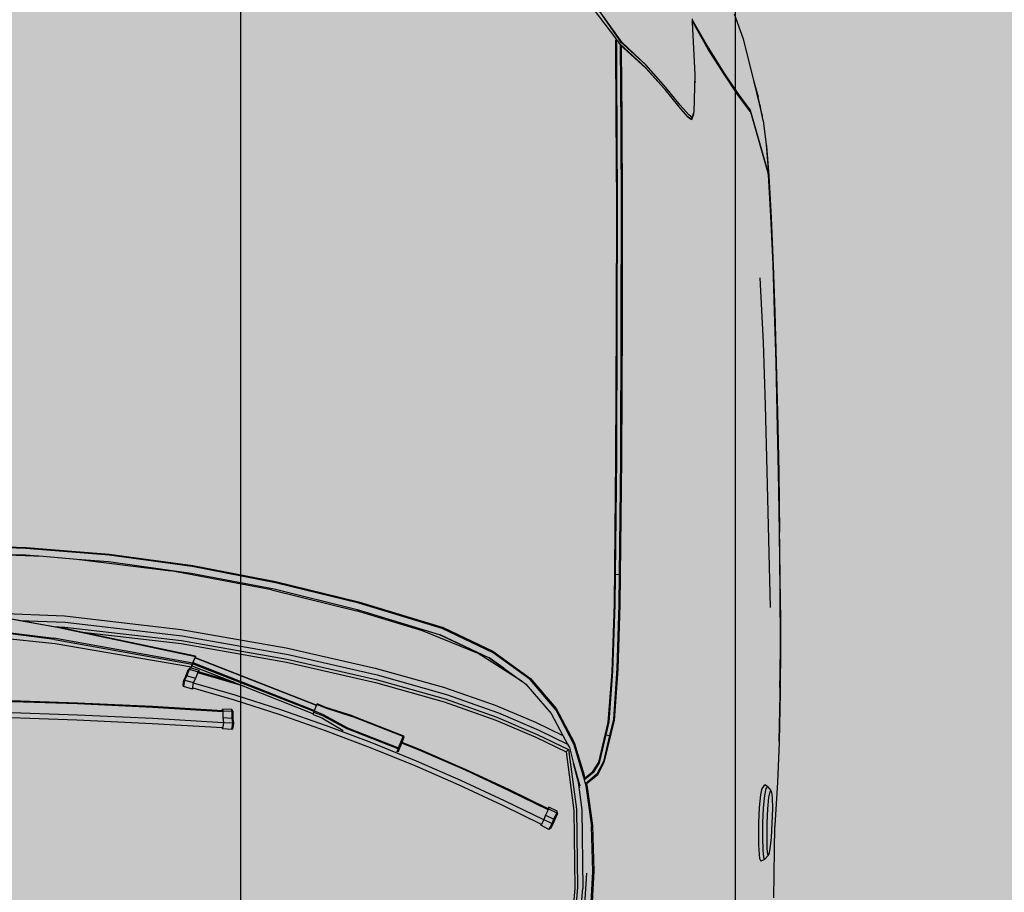
# Model space of a CAD drawing. Units: inches. Extents: x 1884 to 2398, y 474 to 1488.
# Tile 17 of 39: x 2233 to 2275, y 699 to 736. Entities that reach past the tile are written whole.
import ezdxf

# ---------------------------------------------------------------- set-up
doc = ezdxf.new("R2010")
doc.units = ezdxf.units.IN
doc.header["$MEASUREMENT"] = 0
doc.layers.get('0').update_dxf_attribs({"color": 250})
doc.layers.add('A-ANNO-DIMS', color=2, linetype='Continuous', lineweight=18)
doc.layers.add('C-VEHI', color=8, linetype='Continuous', lineweight=18)
doc.layers.add('Edges', color=250, linetype='Continuous')
doc.layers.add('L-PVMT-PATT', color=9, linetype='Continuous', lineweight=13, true_color=0xc7c8ca)
doc.styles.get("Standard").update_dxf_attribs({"font": 'arial.ttf'})
doc.dimstyles.get("Standard").update_dxf_attribs({"dimtxt": 7, "dimasz": 0.18, "dimexe": 0.18, "dimexo": 0.0625, "dimgap": 0.09, "dimtad": 0, "dimtih": 1, "dimtoh": 1, "dimzin": 0, "dimdsep": 46, "dimlunit": 3, "dimtxsty": 'Standard', "dimcen": 0.09, "dimadec": 0, "dimazin": 0, "dimtfac": 1, "dimtofl": 0, "dimtmove": 0, "dimatfit": 3, "dimfxl": 1, "dimtolj": 1, "dimtzin": 0, "dimarcsym": 0})

# ---------------------------------------------------------------- blocks, each defined once
blk = doc.blocks.new('Nissan Qashqai pl')
at = {"layer": 'Edges'}
for p, q in [((8.0713, 12.8205), (8.016, 12.8189)), ((8.0168, 12.8191), (8.0718, 12.8207)), ((8.1249, 12.8218), (8.0713, 12.8205)), ((8.0718, 12.8207), (8.1251, 12.822)), ((8.1901, 12.8232), (8.1249, 12.8218)), ((8.1251, 12.822), (8.1902, 12.8233)), ((8.2094, 12.8235), (8.1901, 12.8232)), ((8.1902, 12.8233), (8.2543, 12.8243)), ((8.2543, 12.8243), (8.2094, 12.8235)), ((8.2543, 12.8243), (8.2094, 12.8235)), ((8.2544, 12.8242), (8.2094, 12.8235)), ((8.2693, 12.8245), (8.2543, 12.8243)), ((8.3166, 12.8249), (8.2544, 12.8242)), ((8.3098, 12.825), (8.2693, 12.8245)), ((8.3159, 12.825), (8.2693, 12.8245)), ((8.3159, 12.825), (8.3098, 12.825)), ((8.3159, 12.825), (8.3163, 12.825)), ((8.3163, 12.825), (8.3657, 12.8252)), ((8.3163, 12.825), (8.3597, 12.8252)), ((8.3764, 12.8251), (8.3166, 12.8249)), ((8.3597, 12.8252), (8.3657, 12.8252)), ((8.3657, 12.8252), (8.3663, 12.8252)), ((8.3663, 12.8252), (8.3747, 12.8252)), ((8.3764, 12.8251), (8.3663, 12.8252)), ((8.3747, 12.8252), (8.3757, 12.8252)), ((8.3757, 12.8252), (8.4282, 12.8249)), ((8.4069, 12.8249), (8.3764, 12.8251)), ((8.4219, 12.8246), (8.4069, 12.8249)), ((8.4292, 12.8248), (8.4069, 12.8249)), ((8.4282, 12.8249), (8.4799, 12.8239)), ((8.4799, 12.8239), (8.4292, 12.8248)), ((8.4799, 12.8239), (8.4811, 12.8239)), ((8.4811, 12.8239), (8.5241, 12.8222)), ((8.5241, 12.8222), (8.5707, 12.8193)), ((7.8676, 12.8123), (7.7998, 12.7928)), ((7.8012, 12.7929), (7.8681, 12.8121)), ((7.8107, 12.8065), (7.8363, 12.8097)), ((7.8363, 12.8097), (7.8676, 12.8123)), ((7.8363, 12.8097), (7.8381, 12.81)), ((7.8381, 12.81), (7.87, 12.8126)), ((7.8676, 12.8123), (7.8681, 12.8121)), ((7.869, 12.8124), (7.8681, 12.8121)), ((7.9137, 12.815), (7.869, 12.8124)), ((7.87, 12.8126), (7.9151, 12.8152)), ((7.9658, 12.8172), (7.9137, 12.815)), ((7.9151, 12.8152), (7.9668, 12.8174)), ((8.016, 12.8189), (7.9658, 12.8172)), ((7.9668, 12.8174), (8.0168, 12.8191)), ((8.1176, 12.8087), (8.1888, 12.8107)), ((8.1888, 12.8107), (8.2622, 12.8125)), ((8.2622, 12.8125), (8.3356, 12.8141)), ((8.5287, 12.8112), (8.5269, 12.8082)), ((8.5287, 12.8112), (8.5331, 12.815)), ((8.5287, 12.8112), (8.531, 12.8095)), ((8.5347, 12.8159), (8.5331, 12.815)), ((8.5331, 12.815), (8.5346, 12.8138)), ((8.5346, 12.8138), (8.5406, 12.8125)), ((8.5407, 12.8167), (8.5347, 12.8159)), ((8.5406, 12.8125), (8.5526, 12.8114)), ((8.5527, 12.8169), (8.5407, 12.8167)), ((8.5526, 12.8114), (8.5681, 12.8107)), ((8.5682, 12.8164), (8.5527, 12.8169)), ((8.5681, 12.8107), (8.5836, 12.8104)), ((8.5837, 12.8154), (8.5682, 12.8164)), ((8.5707, 12.8193), (8.5719, 12.8193)), ((8.6489, 12.8179), (8.5719, 12.8193)), ((8.5836, 12.8104), (8.5957, 12.8107)), ((8.5958, 12.8141), (8.5837, 12.8154)), ((8.5957, 12.8107), (8.6017, 12.8114)), ((8.6018, 12.8129), (8.5958, 12.8141)), ((8.6017, 12.8114), (8.6032, 12.8121)), ((8.6032, 12.8121), (8.6018, 12.8129)), ((8.6073, 12.808), (8.6032, 12.8121)), ((7.7673, 12.7961), (7.8058, 12.8055)), ((7.7673, 12.7961), (7.7848, 12.8012)), ((7.7835, 12.8007), (7.7835, 12.8007)), ((7.8087, 12.8062), (7.7848, 12.8012)), ((7.7865, 12.8013), (7.7866, 12.8013)), ((7.7936, 12.8029), (7.7977, 12.8038)), ((7.8106, 12.8065), (7.8087, 12.8062)), ((7.8106, 12.8065), (7.8107, 12.8065)), ((7.9803, 12.803), (8.05, 12.8066)), ((8.05, 12.8066), (8.1176, 12.8087)), ((8.5322, 12.8047), (8.5269, 12.8082)), ((8.531, 12.8095), (8.5385, 12.8079)), ((8.5322, 12.8047), (8.5375, 12.8036)), ((8.5375, 12.8036), (8.5513, 12.8023)), ((8.5385, 12.8079), (8.5518, 12.8066)), ((8.5513, 12.8023), (8.5678, 12.8016)), ((8.5518, 12.8066), (8.568, 12.8059)), ((8.5678, 12.8016), (8.5844, 12.8014)), ((8.568, 12.8059), (8.5842, 12.8057)), ((8.5842, 12.8057), (8.5974, 12.8061)), ((8.5844, 12.8014), (8.5921, 12.8016)), ((8.5921, 12.8016), (8.6021, 12.8022)), ((8.5974, 12.8061), (8.6049, 12.8069)), ((8.6021, 12.8022), (8.6065, 12.8027)), ((8.6049, 12.8069), (8.6073, 12.808)), ((8.6065, 12.8027), (8.6093, 12.804)), ((8.6073, 12.808), (8.6093, 12.804)), ((7.7223, 12.7851), (7.7673, 12.7961)), ((7.7814, 12.7791), (7.7991, 12.7923)), ((7.7984, 12.7909), (7.7828, 12.7793)), ((7.7976, 12.792), (7.7991, 12.7923)), ((7.8007, 12.7926), (7.7984, 12.7909)), ((7.7991, 12.7923), (7.7998, 12.7928)), ((7.7995, 12.7924), (7.8007, 12.7926)), ((7.8012, 12.7929), (7.8007, 12.7926)), ((7.6953, 12.7753), (7.7223, 12.7851)), ((7.7591, 12.7641), (7.7814, 12.7791)), ((7.7828, 12.7793), (7.7606, 12.7644)), ((7.7325, 12.7476), (7.7591, 12.7641)), ((7.7606, 12.7644), (7.7341, 12.7478)), ((7.7038, 12.731), (7.7325, 12.7476)), ((7.7341, 12.7478), (7.7056, 12.7314)), ((7.701, 12.73), (7.7024, 12.7301)), ((7.7024, 12.7301), (7.7038, 12.731)), ((7.7024, 12.7301), (7.7034, 12.7301)), ((7.7056, 12.7314), (7.7034, 12.7301)), ((7.7034, 12.7301), (7.7048, 12.7302)), ((7.7048, 12.7302), (7.7608, 12.7329)), ((7.7058, 12.7308), (7.7048, 12.7302)), ((7.7608, 12.7329), (7.8014, 12.7318)), ((7.7688, 12.7328), (7.7688, 12.734)), ((7.8045, 12.7263), (7.7938, 12.7171)), ((7.8062, 12.725), (7.7959, 12.7161)), ((7.8014, 12.7318), (7.8022, 12.7316)), ((7.8022, 12.7316), (7.8037, 12.7315)), ((7.8022, 12.7316), (7.8072, 12.73)), ((7.8037, 12.7315), (7.8096, 12.7294)), ((7.8072, 12.73), (7.8045, 12.7263)), ((7.8062, 12.725), (7.8087, 12.7283)), ((7.8066, 12.7254), (7.8062, 12.725)), ((7.8096, 12.7294), (7.8066, 12.7254)), ((7.8072, 12.73), (7.8087, 12.7283)), ((7.7938, 12.7171), (7.7748, 12.7018)), ((7.7959, 12.7161), (7.7772, 12.7011)), ((7.7748, 12.7018), (7.7507, 12.6803)), ((7.753, 12.6794), (7.776, 12.6999)), ((7.776, 12.6999), (7.7539, 12.68)), ((7.7772, 12.7011), (7.776, 12.6999)), ((7.7261, 12.6543), (7.7507, 12.6803)), ((7.753, 12.6794), (7.7281, 12.6524)), ((7.7507, 12.6803), (7.7286, 12.6561)), ((7.7539, 12.68), (7.7324, 12.6565)), ((7.7261, 12.6543), (7.6762, 12.6186)), ((7.6762, 12.6186), (7.7233, 12.6514)), ((7.7281, 12.6524), (7.7232, 12.6486)), ((7.7267, 12.6539), (7.7233, 12.6514)), ((7.7286, 12.6561), (7.7267, 12.6539)), ((7.7299, 12.6537), (7.7281, 12.6524)), ((7.7281, 12.6524), (7.7349, 12.6524)), ((7.7324, 12.6565), (7.7299, 12.6537)), ((7.7299, 12.6537), (7.7334, 12.6537)), ((7.7334, 12.6537), (7.8083, 12.6544)), ((7.7349, 12.6524), (7.768, 12.6527)), ((7.768, 12.6527), (7.7692, 12.6527)), ((7.7692, 12.6527), (7.7844, 12.6528)), ((7.7844, 12.6528), (7.8078, 12.653)), ((7.8078, 12.653), (7.8233, 12.6531)), ((7.8083, 12.6544), (7.904, 12.6547)), ((7.8233, 12.6531), (7.9036, 12.6534)), ((7.9036, 12.6534), (8.0275, 12.6533)), ((7.904, 12.6547), (8.0276, 12.6545)), ((8.0275, 12.6533), (8.1755, 12.6527)), ((8.0276, 12.6545), (8.1753, 12.6539)), ((8.1753, 12.6539), (8.3324, 12.6521)), ((8.1755, 12.6527), (8.3005, 12.6514)), ((8.3005, 12.6514), (8.3002, 12.6474)), ((8.3005, 12.6514), (8.3324, 12.651)), ((8.3324, 12.6521), (8.4022, 12.6498)), ((8.3324, 12.651), (8.4014, 12.6488)), ((7.6771, 12.6135), (7.7215, 12.6473)), ((7.7215, 12.6473), (7.7221, 12.6478)), ((7.7232, 12.6486), (7.7221, 12.6478)), ((7.7245, 12.6486), (7.7232, 12.6486)), ((7.7261, 12.6476), (7.7238, 12.6476)), ((7.7294, 12.6487), (7.7245, 12.6486)), ((7.7279, 12.6477), (7.7261, 12.6476)), ((7.8048, 12.6483), (7.7279, 12.6477)), ((7.731, 12.6487), (7.7294, 12.6487)), ((7.764, 12.6489), (7.731, 12.6487)), ((7.7662, 12.6489), (7.764, 12.6489)), ((7.7811, 12.649), (7.7662, 12.6489)), ((7.7822, 12.649), (7.7811, 12.649)), ((7.8057, 12.6491), (7.7822, 12.649)), ((7.9014, 12.6487), (7.8048, 12.6483)), ((7.8233, 12.6492), (7.8057, 12.6491)), ((7.902, 12.6495), (7.8233, 12.6492)), ((8.0273, 12.6485), (7.9014, 12.6487)), ((8.0275, 12.6493), (7.902, 12.6495)), ((8.1753, 12.6479), (8.0273, 12.6485)), ((8.1754, 12.6487), (8.0275, 12.6493)), ((8.3318, 12.6462), (8.1753, 12.6479)), ((8.3002, 12.6474), (8.1754, 12.6487)), ((8.332, 12.6471), (8.3002, 12.6474)), ((8.4049, 12.6437), (8.3318, 12.6462)), ((8.4042, 12.6447), (8.332, 12.6471)), ((8.4014, 12.6488), (8.4559, 12.6451)), ((8.4022, 12.6498), (8.4571, 12.6459)), ((8.4588, 12.6405), (8.4042, 12.6447)), ((8.4595, 12.6395), (8.4049, 12.6437)), ((8.4559, 12.6451), (8.4736, 12.6409)), ((8.4571, 12.6459), (8.5029, 12.635)), ((8.4729, 12.6372), (8.4588, 12.6405)), ((8.4729, 12.6372), (8.4736, 12.6409)), ((8.4736, 12.6409), (8.5018, 12.6344)), ((8.5025, 12.6293), (8.4595, 12.6395)), ((8.5032, 12.6301), (8.4729, 12.6372)), ((8.5018, 12.6344), (8.5155, 12.6274)), ((8.5125, 12.6231), (8.5025, 12.6293)), ((8.5029, 12.635), (8.5163, 12.6279)), ((8.5132, 12.624), (8.5032, 12.6301)), ((8.5177, 12.617), (8.5125, 12.6231)), ((8.5132, 12.624), (8.5216, 12.6139)), ((8.5155, 12.6274), (8.5258, 12.6151)), ((8.5163, 12.6279), (8.5237, 12.6189)), ((8.5237, 12.6189), (8.5259, 12.6162)), ((8.5294, 12.6167), (8.5706, 12.6226)), ((8.5304, 12.6157), (8.5715, 12.6215)), ((8.5706, 12.6226), (8.6197, 12.6241)), ((8.6203, 12.6229), (8.5715, 12.6215)), ((8.6197, 12.6241), (8.6683, 12.6215)), ((8.6203, 12.6229), (8.6204, 12.6229)), ((8.6721, 12.6201), (8.6204, 12.6229)), ((8.4814, 12.6029), (8.5166, 12.6135)), ((8.5216, 12.6139), (8.4838, 12.6027)), ((8.5039, 12.6023), (8.528, 12.6088)), ((8.5166, 12.6135), (8.5197, 12.6145)), ((8.5197, 12.6145), (8.5177, 12.617)), ((8.5197, 12.6145), (8.5216, 12.6139)), ((8.5258, 12.6151), (8.5216, 12.6139)), ((8.5216, 12.6068), (8.5538, 12.6111)), ((8.5301, 12.609), (8.5216, 12.6068)), ((8.5259, 12.6162), (8.5258, 12.6151)), ((8.5258, 12.6151), (8.5304, 12.6157)), ((8.5259, 12.6162), (8.5294, 12.6167)), ((8.5304, 12.6157), (8.5304, 12.6157)), ((8.5538, 12.6111), (8.6387, 12.6123)), ((8.622, 12.6161), (8.6699, 12.6132)), ((8.6721, 12.6093), (8.6387, 12.6123)), ((8.4444, 12.5834), (8.4814, 12.6029)), ((8.4838, 12.6027), (8.4462, 12.5833)), ((8.4831, 12.5957), (8.4867, 12.5977)), ((8.4867, 12.5977), (8.5039, 12.6023)), ((8.4889, 12.5969), (8.5531, 12.6055)), ((8.4914, 12.5942), (8.5544, 12.6026)), ((8.5216, 12.6068), (8.5039, 12.6023)), ((8.5531, 12.6055), (8.6375, 12.6066)), ((8.5544, 12.6026), (8.6386, 12.6037)), ((8.6375, 12.6066), (8.7481, 12.5968)), ((8.6386, 12.6037), (8.7491, 12.594)), ((8.4499, 12.5782), (8.4737, 12.5908)), ((8.4594, 12.5611), (8.4737, 12.5908)), ((8.468, 12.5648), (8.4831, 12.5957)), ((8.4725, 12.563), (8.4889, 12.5969)), ((8.4737, 12.5908), (8.4831, 12.5957)), ((8.4756, 12.5615), (8.4914, 12.5942)), ((8.4914, 12.5942), (8.4889, 12.5969)), ((8.4122, 12.5558), (8.4444, 12.5834)), ((8.4462, 12.5833), (8.4134, 12.5554)), ((8.4183, 12.5508), (8.4499, 12.5782)), ((8.5554, 12.5847), (8.551, 12.5757)), ((8.5529, 12.5751), (8.5572, 12.5841)), ((8.5574, 12.5849), (8.5554, 12.5847)), ((8.5572, 12.5841), (8.5554, 12.5847)), ((8.5639, 12.581), (8.5572, 12.5841)), ((8.5574, 12.5849), (8.5584, 12.5846)), ((8.5582, 12.5845), (8.5574, 12.5849)), ((8.5584, 12.5846), (8.5649, 12.5816)), ((8.5595, 12.572), (8.5639, 12.581)), ((8.5687, 12.5791), (8.5639, 12.581)), ((8.5644, 12.5701), (8.5687, 12.5791)), ((8.5649, 12.5816), (8.5693, 12.5799)), ((8.5687, 12.5791), (8.5693, 12.5799)), ((8.5749, 12.5757), (8.5687, 12.5791)), ((8.5693, 12.5799), (8.5739, 12.5774)), ((8.5739, 12.5774), (8.5749, 12.5757)), ((8.5527, 12.5749), (8.5323, 12.5332)), ((8.5537, 12.5747), (8.5332, 12.5329)), ((8.5647, 12.57), (8.5441, 12.5279)), ((8.5487, 12.5256), (8.5692, 12.5674)), ((8.5527, 12.5749), (8.551, 12.5757)), ((8.551, 12.5757), (8.5528, 12.5751)), ((8.5528, 12.5751), (8.5527, 12.5749)), ((8.5528, 12.5751), (8.5529, 12.5751)), ((8.5529, 12.5751), (8.5537, 12.5747)), ((8.5537, 12.5747), (8.5595, 12.572)), ((8.5595, 12.572), (8.5644, 12.5701)), ((8.5644, 12.5701), (8.5647, 12.57)), ((8.5647, 12.57), (8.5692, 12.5675)), ((8.5692, 12.5674), (8.5692, 12.5675)), ((8.5692, 12.5675), (8.5705, 12.5668)), ((8.5705, 12.5668), (8.5692, 12.5674)), ((8.5749, 12.5757), (8.5705, 12.5668)), ((8.3826, 12.5151), (8.4122, 12.5558)), ((8.4134, 12.5554), (8.3844, 12.5157)), ((8.4411, 12.5178), (8.4594, 12.5611)), ((8.4493, 12.5212), (8.468, 12.5648)), ((8.454, 12.5196), (8.4725, 12.563)), ((8.4571, 12.5184), (8.4756, 12.5615)), ((8.4154, 12.5468), (8.3852, 12.4994)), ((8.3901, 12.5113), (8.4154, 12.5468)), ((8.4011, 12.5269), (8.4154, 12.5468)), ((8.4156, 12.547), (8.4154, 12.5468)), ((8.4156, 12.547), (8.4183, 12.5508)), ((8.4011, 12.5269), (8.3901, 12.5113)), ((8.3904, 12.512), (8.4011, 12.5269)), ((8.5323, 12.5332), (8.5103, 12.4859)), ((8.5332, 12.5329), (8.5112, 12.4856)), ((8.5441, 12.5279), (8.5222, 12.4807)), ((8.5269, 12.4785), (8.5487, 12.5256)), ((8.3573, 12.4618), (8.3826, 12.5151)), ((8.3844, 12.5157), (8.3582, 12.4606)), ((8.4217, 12.4622), (8.4411, 12.5178)), ((8.4296, 12.4651), (8.4493, 12.5212)), ((8.4343, 12.4637), (8.454, 12.5196)), ((8.4375, 12.4627), (8.4571, 12.5184)), ((8.3646, 12.4572), (8.39, 12.5111)), ((8.3648, 12.4579), (8.39, 12.5111)), ((8.39, 12.5111), (8.3852, 12.4994)), ((8.39, 12.5111), (8.3901, 12.5113)), ((8.3901, 12.5113), (8.3904, 12.512)), ((8.3852, 12.4994), (8.3608, 12.4393)), ((8.5103, 12.4859), (8.4895, 12.4381)), ((8.5112, 12.4856), (8.4904, 12.4377)), ((8.5222, 12.4807), (8.5014, 12.4329)), ((8.5062, 12.431), (8.5269, 12.4785)), ((8.3296, 12.3703), (8.3573, 12.4618)), ((8.3582, 12.4606), (8.3311, 12.3708)), ((8.4009, 12.3883), (8.4217, 12.4622)), ((8.4084, 12.3907), (8.4296, 12.4651)), ((8.4133, 12.3896), (8.4343, 12.4637)), ((8.4165, 12.3888), (8.4375, 12.4627)), ((8.3377, 12.3689), (8.3646, 12.4572)), ((8.3646, 12.4572), (8.3648, 12.4579)), ((8.3648, 12.4579), (8.3648, 12.4579)), ((8.3608, 12.4393), (8.3392, 12.3684)), ((8.3608, 12.4393), (8.3608, 12.4393)), ((8.4895, 12.4381), (8.4811, 12.4174)), ((8.5014, 12.4329), (8.4817, 12.3847)), ((8.4904, 12.4377), (8.482, 12.4171)), ((8.4866, 12.3829), (8.5062, 12.431)), ((8.4526, 12.3639), (8.4742, 12.4188)), ((8.4747, 12.4185), (8.4532, 12.3636)), ((8.4742, 12.4188), (8.4754, 12.4193)), ((8.4747, 12.4185), (8.4742, 12.4188)), ((8.4754, 12.4193), (8.4747, 12.4185)), ((8.4869, 12.4136), (8.4747, 12.4185)), ((8.4754, 12.4193), (8.4876, 12.4144)), ((8.4791, 12.4183), (8.4754, 12.4193)), ((8.4811, 12.4174), (8.4791, 12.4183)), ((8.482, 12.4171), (8.4811, 12.4174)), ((8.4912, 12.4133), (8.482, 12.4171)), ((8.4654, 12.3587), (8.4869, 12.4136)), ((8.4881, 12.4131), (8.4666, 12.3582)), ((8.4869, 12.4136), (8.4876, 12.4144)), ((8.4881, 12.4131), (8.4869, 12.4136)), ((8.4876, 12.4144), (8.4912, 12.4133)), ((8.4876, 12.4144), (8.4881, 12.4131)), ((8.4914, 12.4121), (8.4881, 12.4131)), ((8.4913, 12.4133), (8.4912, 12.4133)), ((8.4913, 12.4132), (8.4913, 12.4133)), ((8.3792, 12.2926), (8.4009, 12.3883)), ((8.3864, 12.2945), (8.4084, 12.3907)), ((8.3913, 12.2935), (8.4133, 12.3896)), ((8.3945, 12.2929), (8.4165, 12.3888)), ((8.4817, 12.3847), (8.4633, 12.3359)), ((8.4683, 12.3345), (8.4866, 12.3829)), ((8.3076, 12.281), (8.3296, 12.3703)), ((8.3311, 12.3708), (8.3089, 12.2811)), ((8.3157, 12.2795), (8.3377, 12.3689)), ((8.3166, 12.2767), (8.3392, 12.3684)), ((8.4526, 12.3639), (8.4434, 12.3353)), ((8.4439, 12.335), (8.4532, 12.3636)), ((8.4509, 12.3322), (8.4654, 12.3587)), ((8.4521, 12.3317), (8.4666, 12.3582)), ((8.4547, 12.3309), (8.4682, 12.3538)), ((8.4434, 12.3353), (8.4397, 12.326)), ((8.4403, 12.3257), (8.4439, 12.335)), ((8.4633, 12.3359), (8.4461, 12.2868)), ((8.4472, 12.3229), (8.4509, 12.3322)), ((8.4512, 12.2856), (8.4683, 12.3345)), ((8.3894, 12.1944), (8.4409, 12.3255)), ((8.4415, 12.3252), (8.3899, 12.1941)), ((8.3951, 12.192), (8.4467, 12.3231)), ((8.4479, 12.3226), (8.3963, 12.1915)), ((8.4209, 12.2475), (8.4502, 12.3219)), ((8.4403, 12.3257), (8.4397, 12.326)), ((8.4409, 12.3255), (8.4403, 12.3257)), ((8.4415, 12.3252), (8.4409, 12.3255)), ((8.4467, 12.3231), (8.4415, 12.3252)), ((8.4472, 12.3229), (8.4467, 12.3231)), ((8.4479, 12.3226), (8.4472, 12.3229)), ((8.4484, 12.3224), (8.4479, 12.3226)), ((8.4484, 12.3224), (8.4521, 12.3317)), ((8.4502, 12.3219), (8.4484, 12.3224)), ((8.4511, 12.3216), (8.4502, 12.3219)), ((8.4511, 12.3216), (8.4547, 12.3309)), ((8.3593, 12.1791), (8.3792, 12.2926)), ((8.3662, 12.1803), (8.3864, 12.2945)), ((8.3713, 12.1796), (8.3913, 12.2935)), ((8.3745, 12.1792), (8.3945, 12.2929)), ((8.2905, 12.1918), (8.3076, 12.281)), ((8.3089, 12.2811), (8.2916, 12.1913)), ((8.2985, 12.1901), (8.3157, 12.2795)), ((8.4461, 12.2868), (8.4302, 12.2373)), ((8.4353, 12.2363), (8.4512, 12.2856)), ((8.3166, 12.2767), (8.296, 12.168)), ((8.4163, 12.2359), (8.4209, 12.2475)), ((8.4209, 12.2475), (8.4191, 12.2418)), ((8.4191, 12.2418), (8.4061, 12.1973)), ((8.4302, 12.2373), (8.4171, 12.1926)), ((8.3986, 12.1908), (8.4163, 12.2359)), ((8.4163, 12.2359), (8.4052, 12.1979)), ((8.4224, 12.1919), (8.4353, 12.2363)), ((8.4457, 12.2337), (8.4452, 12.2238)), ((8.4475, 12.2348), (8.4457, 12.2337)), ((8.4476, 12.2341), (8.4457, 12.2337)), ((8.4471, 12.2242), (8.4476, 12.2341)), ((8.4475, 12.2348), (8.4484, 12.235)), ((8.4555, 12.2348), (8.4475, 12.2348)), ((8.4549, 12.2341), (8.4476, 12.2341)), ((8.4484, 12.235), (8.4557, 12.235)), ((8.4544, 12.2242), (8.4549, 12.2341)), ((8.46, 12.2348), (8.4549, 12.2341)), ((8.4557, 12.235), (8.4603, 12.2357)), ((8.4595, 12.2249), (8.46, 12.2348)), ((8.46, 12.2348), (8.4603, 12.2357)), ((8.4671, 12.2337), (8.46, 12.2348)), ((8.4603, 12.2357), (8.4655, 12.2348)), ((8.4655, 12.2348), (8.4671, 12.2337)), ((8.4671, 12.2337), (8.4666, 12.2237)), ((8.4471, 12.2238), (8.4425, 12.1485)), ((8.448, 12.2241), (8.4435, 12.1487)), ((8.4452, 12.2238), (8.4471, 12.2242)), ((8.4471, 12.2238), (8.4452, 12.2238)), ((8.4471, 12.2242), (8.4544, 12.2242)), ((8.4471, 12.2239), (8.4471, 12.2238)), ((8.4544, 12.2242), (8.4595, 12.2249)), ((8.4601, 12.2247), (8.4555, 12.1488)), ((8.4595, 12.2249), (8.4666, 12.2237)), ((8.4607, 12.1481), (8.4652, 12.2237)), ((8.4652, 12.2237), (8.4652, 12.2238)), ((8.4666, 12.2237), (8.4652, 12.2237)), ((8.3887, 12.1946), (8.3575, 12.0475)), ((8.3882, 12.1948), (8.3618, 12.07)), ((8.3887, 12.1946), (8.3882, 12.1948)), ((8.3882, 12.1948), (8.3894, 12.1944)), ((8.3894, 12.1944), (8.3887, 12.1946)), ((8.3894, 12.1944), (8.3894, 12.1944)), ((8.3894, 12.1944), (8.3899, 12.1941)), ((8.3899, 12.1941), (8.3951, 12.192)), ((8.4035, 12.1986), (8.4007, 12.189)), ((8.4023, 12.1879), (8.4052, 12.1975)), ((8.4052, 12.1975), (8.4035, 12.1986)), ((8.4035, 12.1986), (8.4052, 12.1979)), ((8.4052, 12.1979), (8.4052, 12.1978)), ((8.412, 12.195), (8.4052, 12.1975)), ((8.4092, 12.1855), (8.412, 12.195)), ((8.4167, 12.1925), (8.412, 12.195)), ((8.2781, 12.1018), (8.2905, 12.1918)), ((8.2916, 12.1913), (8.2793, 12.1016)), ((8.2862, 12.1008), (8.2985, 12.1901)), ((8.3957, 12.1917), (8.3688, 12.0419)), ((8.3702, 12.0427), (8.3969, 12.1913)), ((8.3746, 12.0435), (8.3995, 12.1905)), ((8.3951, 12.192), (8.3963, 12.1915)), ((8.3957, 12.1917), (8.3951, 12.192)), ((8.3969, 12.1913), (8.3957, 12.1917)), ((8.3963, 12.1915), (8.3986, 12.1908)), ((8.3995, 12.1905), (8.3969, 12.1913)), ((8.3995, 12.1905), (8.3986, 12.1908)), ((8.4007, 12.189), (8.4023, 12.1879)), ((8.4007, 12.189), (8.402, 12.1874)), ((8.4028, 12.1868), (8.402, 12.1874)), ((8.402, 12.1874), (8.4027, 12.1871)), ((8.4023, 12.1879), (8.4092, 12.1855)), ((8.4097, 12.1844), (8.4028, 12.1868)), ((8.4092, 12.1855), (8.4139, 12.1829)), ((8.4139, 12.1821), (8.4097, 12.1844)), ((8.4139, 12.1829), (8.4167, 12.1925)), ((8.4237, 12.1914), (8.4167, 12.1925)), ((8.4237, 12.1914), (8.4209, 12.1819)), ((8.4223, 12.1918), (8.4224, 12.1919)), ((8.4224, 12.1919), (8.4237, 12.1914)), ((8.3448, 12.0536), (8.3593, 12.1791)), ((8.3516, 12.0542), (8.3662, 12.1803)), ((8.3567, 12.0538), (8.3713, 12.1796)), ((8.3618, 12.07), (8.3745, 12.1792)), ((8.4139, 12.1829), (8.4209, 12.1819)), ((8.4139, 12.1821), (8.4139, 12.1829)), ((8.4191, 12.1813), (8.4139, 12.1821)), ((8.4209, 12.1819), (8.4191, 12.1813)), ((8.2834, 12.0669), (8.296, 12.168)), ((8.4425, 12.1485), (8.4387, 12.0674)), ((8.4435, 12.1487), (8.4397, 12.0674)), ((8.4555, 12.1488), (8.4517, 12.0674)), ((8.4568, 12.0669), (8.4607, 12.1481)), ((8.2708, 12.0123), (8.2781, 12.1018)), ((8.2793, 12.1016), (8.2719, 12.0118)), ((8.2834, 12.0669), (8.2862, 12.1008)), ((8.2804, 12.0305), (8.2834, 12.0669)), ((8.3618, 12.07), (8.3574, 12.0489)), ((8.4387, 12.0674), (8.4359, 11.9861)), ((8.4397, 12.0674), (8.4369, 11.9861)), ((8.4517, 12.0674), (8.4489, 11.9858)), ((8.4541, 11.9857), (8.4568, 12.0669)), ((8.3575, 12.0475), (8.3104, 11.7881)), ((8.3406, 11.9567), (8.3448, 12.0536)), ((8.3495, 12.0053), (8.3516, 12.0542)), ((8.3562, 12.0421), (8.3567, 12.0538)), ((8.3562, 12.0421), (8.3574, 12.0489)), ((8.336, 11.7828), (8.3688, 12.0419)), ((8.3702, 12.0427), (8.3374, 11.7826)), ((8.3495, 12.0053), (8.3562, 12.0421)), ((8.3565, 11.8707), (8.3746, 12.0435)), ((8.2765, 11.9273), (8.2804, 12.0305)), ((8.2788, 12.0114), (8.2804, 12.0305)), ((8.2682, 11.9221), (8.2708, 12.0123)), ((8.2719, 12.0118), (8.2695, 11.9221)), ((8.2765, 11.9273), (8.2788, 12.0114)), ((8.3406, 11.9567), (8.3495, 12.0053))]:
    blk.add_line(p, q, dxfattribs=at)
blk = doc.blocks.new('car')
blk.add_blockref('Nissan Qashqai pl', (-9.7433, -11.9151))
blk = doc.blocks.new('carr')
blk.add_blockref('car', (0.5124, -0.007))
blk = doc.blocks.new('*D23')
at = {"layer": 'A-ANNO-DIMS', "color": 0, "lineweight": -2, "transparency": 16777216}
for p, q in [((2272.304, 752.812), (2298.291, 752.812)), ((2298.111, 752.632), (2298.111, 670.29)), ((2298.111, 580.529), (2298.111, 662.871)), ((2272.304, 580.349), (2298.291, 580.349))]:
    blk.add_line(p, q, dxfattribs=at)
at = {"layer": 'A-ANNO-DIMS', "color": 0, "lineweight": 100, "transparency": 16777216}
for points in [[(2298.081, 752.632), (2298.141, 752.632), (2298.111, 752.812)], [(2298.081, 580.529), (2298.141, 580.529), (2298.111, 580.349)]]:
    blk.add_solid(points, dxfattribs=at)
at = {"layer": 'Defpoints', "color": 0, "lineweight": 100, "transparency": 16777216}
for p in [(2272.242, 752.812), (2272.242, 580.349), (2298.111, 580.349)]:
    blk.add_point(p, dxfattribs=at)
at = {"layer": 'A-ANNO-DIMS', "color": 0, "transparency": 16777216, "insert": (2298.111, 666.58), "char_height": 7, "attachment_point": 5}
blk.add_mtext('\\A1;CAR 14\'-4 1/2" TYP.', dxfattribs=at)
blk = doc.blocks.new('*D44')
at = {"layer": 'A-ANNO-DIMS', "color": 0, "lineweight": -2, "transparency": 16777216}
for p, q in [((2209.755, 1247.822), (2209.755, 484.005)), ((2230.029, 1247.822), (2230.029, 484.005)), ((2209.935, 484.185), (2229.849, 484.185)), ((2230.029, 484.185), (2230.209, 484.185))]:
    blk.add_line(p, q, dxfattribs=at)
at = {"layer": 'A-ANNO-DIMS', "color": 0, "lineweight": 100, "transparency": 16777216}
for points in [[(2209.935, 484.215), (2209.935, 484.155), (2209.755, 484.185)], [(2229.849, 484.215), (2229.849, 484.155), (2230.029, 484.185)]]:
    blk.add_solid(points, dxfattribs=at)
at = {"layer": 'Defpoints', "color": 0, "lineweight": 100, "transparency": 16777216}
for p in [(2209.755, 1247.885), (2230.029, 1247.885), (2230.029, 484.185)]:
    blk.add_point(p, dxfattribs=at)
at = {"layer": 'A-ANNO-DIMS', "color": 0, "transparency": 16777216, "insert": (2247.429, 484.185), "char_height": 7, "attachment_point": 5}
blk.add_mtext('\\A1;1\'-8 1/2"', dxfattribs=at)
blk = doc.blocks.new('*D45')
at = {"layer": 'A-ANNO-DIMS', "color": 0, "lineweight": -2, "transparency": 16777216}
for p, q in [((2242.617, 1322.822), (2242.617, 484.005)), ((2263.617, 1322.822), (2263.617, 484.005)), ((2242.797, 484.185), (2244.052, 484.185)), ((2263.437, 484.185), (2262.181, 484.185))]:
    blk.add_line(p, q, dxfattribs=at)
at = {"layer": 'A-ANNO-DIMS', "color": 0, "lineweight": 100, "transparency": 16777216}
for points in [[(2242.797, 484.215), (2242.797, 484.155), (2242.617, 484.185)], [(2263.437, 484.215), (2263.437, 484.155), (2263.617, 484.185)]]:
    blk.add_solid(points, dxfattribs=at)
at = {"layer": 'Defpoints', "color": 0, "lineweight": 100, "transparency": 16777216}
for p in [(2242.617, 1322.885), (2263.617, 1322.885), (2263.617, 484.185)]:
    blk.add_point(p, dxfattribs=at)
at = {"layer": 'A-ANNO-DIMS', "color": 0, "transparency": 16777216, "insert": (2253.117, 484.185), "char_height": 7, "attachment_point": 5}
blk.add_mtext('\\A1;1\'-9"', dxfattribs=at)

msp = doc.modelspace()

# ---------------------------------------------------------------- hatches: boundary and pattern name
at = {"layer": 'L-PVMT-PATT'}
h = msp.add_hatch(color=256, dxfattribs=at)
h.dxf.hatch_style = 1
h.paths.add_polyline_path([(2387.529, 769.966), (2351.529, 769.966), (2238.447, 769.966), (2238.447, 762.15), (2238.447, 754.445), (2126.529, 754.445), (2126.529, 676.183), (2134.868, 676.183), (2142.673, 676.183), (2142.673, 646.578), (2134.868, 646.578), (2126.529, 646.578), (2126.529, 640.17), (2387.529, 640.17)])
h.paths.add_polyline_path([(2387.529, 631.385), (2303.086, 631.385), (2303.086, 615.671), (2387.529, 615.671)])
h.paths.add_polyline_path([(2387.529, 640.17), (2126.529, 640.17), (2126.529, 631.385), (2387.529, 631.385)])
h.paths.add_polyline_path([(2393.529, 604.13), (2387.529, 604.13), (2387.529, 615.671), (2303.086, 615.671), (2303.086, 607.943), (2249.649, 607.943), (2126.529, 607.943), (2126.529, 533.885), (2393.529, 533.885)])
h.paths.add_polyline_path([(2257.825, 611.008), (2257.83, 611.337), (2257.915, 616.493), (2258.021, 621.805), (2258.146, 627.274), (2258.252, 631.385), (2126.529, 631.385), (2126.529, 611.008)])
h.paths.add_polyline_path([(2258.892, 611.285), (2258.888, 611.008), (2300.247, 611.008), (2300.247, 631.385), (2259.314, 631.385), (2259.206, 627.173), (2259.081, 621.72), (2258.976, 616.424)])

# ---------------------------------------------------------------- block references
at = {"layer": 'C-VEHI', "xscale": 39.37007874015748, "yscale": 39.37007874015748, "zscale": 39.37007874015748, "rotation": 270}
msp.add_blockref('carr', (2229.977, 676.232), dxfattribs=at)

# ---------------------------------------------------------------- dimensions: what is measured, and where the dimension line sits
at = {"layer": 'A-ANNO-DIMS'}
for base, p1, p2, picture, middle in [((2263.617, 484.185), (2242.617, 1322.885), (2263.617, 1322.885), '*D45', (2253.117, 484.185)), ((2230.029, 484.185), (2209.755, 1247.885), (2230.029, 1247.885), '*D44', (2247.429, 484.185))]:
    dim = msp.add_linear_dim(base=base, p1=p1, p2=p2, dimstyle='Standard', override={"dimdec": 1, "dimlfac": 1, "dimrnd": 0, "dimzin": 1, "dimdsep": 46, "dimlunit": 4, "dimfrac": 2}, dxfattribs=at)
    dim.commit()
    dim.dimension.update_dxf_attribs({"geometry": picture, "text_midpoint": middle})
dim = msp.add_linear_dim(base=(2298.111, 580.349), p1=(2272.242, 752.812), p2=(2272.242, 580.349), angle=270, text='CAR <> TYP.', dimstyle='Standard', override={"dimdec": 1, "dimlfac": 1, "dimrnd": 0, "dimzin": 1, "dimdsep": 46, "dimlunit": 4, "dimfrac": 2}, dxfattribs=at)
dim.commit()
dim.dimension.update_dxf_attribs({"geometry": '*D23', "text_midpoint": (2298.111, 666.58)})

doc.saveas('drawing.dxf')
